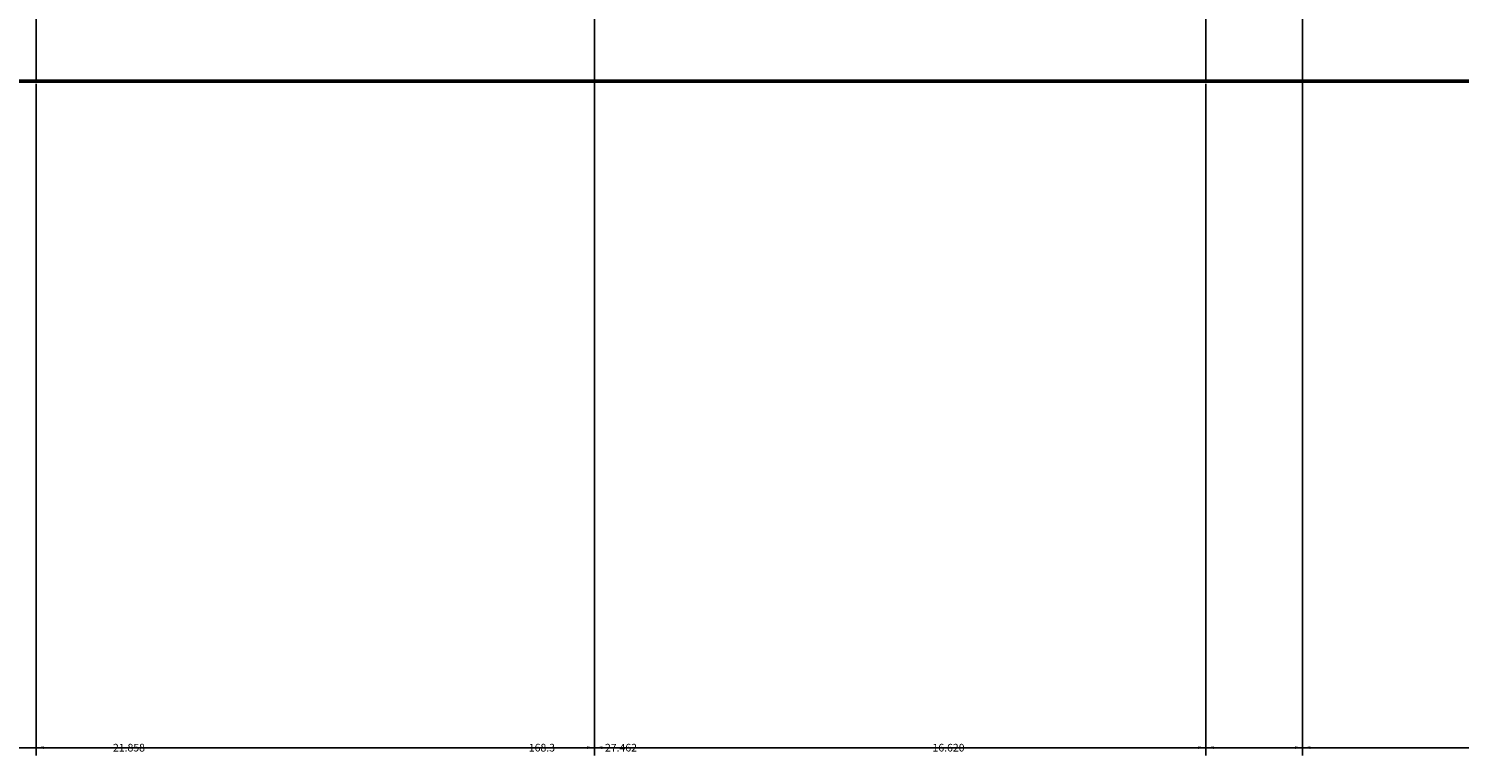
# Model space of a CAD drawing. Units: inches. Extents: x -117 to 121, y -77 to 40.
# Tile 19 of 45: x -6 to 28, y -77 to -60. Entities that reach past the tile are written whole.
import ezdxf

# ---------------------------------------------------------------- set-up
doc = ezdxf.new("R2010")
doc.units = ezdxf.units.IN
doc.header["$MEASUREMENT"] = 0
for name, color, linetype, lineweight in [('A-ANNO-DIMS', 2, 'Continuous', 18), ('A-ELEV', 7, 'Continuous', 25), ('A-ELEV-GRND', 7, 'Continuous', 50)]:
    doc.layers.add(name, color=color, linetype=linetype, lineweight=lineweight)
doc.styles.get("Standard").update_dxf_attribs({"font": 'arial.ttf'})
doc.dimstyles.get("Standard").update_dxf_attribs({"dimtxt": 0.18, "dimasz": 0.18, "dimexe": 0.18, "dimexo": 0.0625, "dimgap": 0.09, "dimtad": 0, "dimtih": 1, "dimtoh": 1, "dimdec": 4, "dimzin": 0, "dimdsep": 46, "dimtxsty": 'Standard', "dimcen": 0.09, "dimadec": 0, "dimazin": 0, "dimtfac": 1, "dimtdec": 4, "dimtofl": 0, "dimtmove": 0, "dimatfit": 3, "dimfxl": 1, "dimtolj": 1, "dimtzin": 0, "dimarcsym": 0})

# ---------------------------------------------------------------- blocks, each defined once
blk = doc.blocks.new('*D7')
at = {"layer": 'A-ANNO-DIMS', "color": 0, "lineweight": -2, "transparency": 16777216}
for p, q in [((-77.763, -61.431), (-77.763, -77.193)), ((90.549, -61.438), (90.549, -77.193)), ((-77.583, -77.013), (6.008, -77.013)), ((90.369, -77.013), (6.778, -77.013))]:
    blk.add_line(p, q, dxfattribs=at)
at = {"layer": 'A-ANNO-DIMS', "color": 0, "transparency": 16777216}
for points in [[(-77.583, -76.983), (-77.583, -77.043), (-77.763, -77.013)], [(90.369, -76.983), (90.369, -77.043), (90.549, -77.013)]]:
    blk.add_solid(points, dxfattribs=at)
at = {"layer": 'Defpoints', "color": 0, "transparency": 16777216}
for p in [(-77.763, -61.369), (90.549, -61.376), (90.549, -77.013)]:
    blk.add_point(p, dxfattribs=at)
at = {"layer": 'A-ANNO-DIMS', "color": 0, "transparency": 16777216, "insert": (6.393, -77.013), "char_height": 0.18, "attachment_point": 5}
blk.add_mtext('\\A1;168.3', dxfattribs=at)
blk = doc.blocks.new('*D13')
at = {"layer": 'A-ANNO-DIMS', "color": 0, "lineweight": -2, "transparency": 16777216}
for p, q in [((-2.663, 27.063), (-117.024, 27.063)), ((-116.844, 26.883), (-116.844, -16.974)), ((-116.844, -61.196), (-116.844, -17.338)), ((-106.096, -61.376), (-117.024, -61.376))]:
    blk.add_line(p, q, dxfattribs=at)
at = {"layer": 'A-ANNO-DIMS', "color": 0, "transparency": 16777216}
for points in [[(-116.874, 26.883), (-116.814, 26.883), (-116.844, 27.063)], [(-116.874, -61.196), (-116.814, -61.196), (-116.844, -61.376)]]:
    blk.add_solid(points, dxfattribs=at)
at = {"layer": 'Defpoints', "color": 0, "transparency": 16777216}
for p in [(-2.6, 27.063), (-116.844, -61.376), (-106.034, -61.376)]:
    blk.add_point(p, dxfattribs=at)
at = {"layer": 'A-ANNO-DIMS', "color": 0, "transparency": 16777216, "insert": (-116.844, -17.156), "char_height": 0.18, "attachment_point": 5}
blk.add_mtext('\\A1;88.44', dxfattribs=at)
blk = doc.blocks.new('*D25')
at = {"layer": 'A-ANNO-DIMS', "color": 0, "lineweight": -2, "transparency": 16777216}
for p, q in [((-5.482, -61.438), (-5.482, -77.193)), ((21.98, -61.438), (21.98, -77.193)), ((-5.302, -77.013), (7.784, -77.013)), ((21.8, -77.013), (8.713, -77.013))]:
    blk.add_line(p, q, dxfattribs=at)
at = {"layer": 'A-ANNO-DIMS', "color": 0, "transparency": 16777216}
for points in [[(-5.302, -76.983), (-5.302, -77.043), (-5.482, -77.013)], [(21.8, -76.983), (21.8, -77.043), (21.98, -77.013)]]:
    blk.add_solid(points, dxfattribs=at)
at = {"layer": 'Defpoints', "color": 0, "transparency": 16777216}
for p in [(-5.482, -61.376), (21.98, -61.376), (21.98, -77.013)]:
    blk.add_point(p, dxfattribs=at)
at = {"layer": 'A-ANNO-DIMS', "color": 0, "transparency": 16777216, "insert": (8.249, -77.013), "char_height": 0.18, "attachment_point": 5}
blk.add_mtext('\\A1;27.462', dxfattribs=at)
blk = doc.blocks.new('*D26')
at = {"layer": 'A-ANNO-DIMS', "color": 0, "lineweight": -2, "transparency": 16777216}
for p, q in [((21.98, -61.438), (21.98, -77.193)), ((40.68, -61.438), (40.68, -77.193)), ((22.16, -77.013), (30.892, -77.013)), ((40.5, -77.013), (31.768, -77.013))]:
    blk.add_line(p, q, dxfattribs=at)
at = {"layer": 'A-ANNO-DIMS', "color": 0, "transparency": 16777216}
for points in [[(22.16, -76.983), (22.16, -77.043), (21.98, -77.013)], [(40.5, -76.983), (40.5, -77.043), (40.68, -77.013)]]:
    blk.add_solid(points, dxfattribs=at)
at = {"layer": 'Defpoints', "color": 0, "transparency": 16777216}
for p in [(21.98, -61.376), (40.68, -61.376), (40.68, -77.013)]:
    blk.add_point(p, dxfattribs=at)
at = {"layer": 'A-ANNO-DIMS', "color": 0, "transparency": 16777216, "insert": (31.33, -77.013), "char_height": 0.18, "attachment_point": 5}
blk.add_mtext('\\A1;18.701', dxfattribs=at)
blk = doc.blocks.new('*D56')
at = {"layer": 'A-ANNO-DIMS', "color": 0, "lineweight": -2, "transparency": 16777216}
for p, q in [((-14.23, -7.853), (-14.23, -77.193)), ((7.628, -8.105), (7.628, -77.193)), ((-14.05, -77.013), (-3.766, -77.013)), ((7.448, -77.013), (-2.835, -77.013))]:
    blk.add_line(p, q, dxfattribs=at)
at = {"layer": 'A-ANNO-DIMS', "color": 0, "transparency": 16777216}
for points in [[(-14.05, -76.983), (-14.05, -77.043), (-14.23, -77.013)], [(7.448, -76.983), (7.448, -77.043), (7.628, -77.013)]]:
    blk.add_solid(points, dxfattribs=at)
at = {"layer": 'Defpoints', "color": 0, "transparency": 16777216}
for p in [(-14.23, -7.791), (7.628, -8.042), (7.628, -77.013)]:
    blk.add_point(p, dxfattribs=at)
at = {"layer": 'A-ANNO-DIMS', "color": 0, "transparency": 16777216, "insert": (-3.301, -77.013), "char_height": 0.18, "attachment_point": 5}
blk.add_mtext('\\A1;21.858', dxfattribs=at)
blk = doc.blocks.new('*D57')
at = {"layer": 'A-ANNO-DIMS', "color": 0, "lineweight": -2, "transparency": 16777216}
for p, q in [((7.628, -8.105), (7.628, -77.193)), ((24.248, -8.105), (24.248, -77.193)), ((7.808, -77.013), (15.483, -77.013)), ((24.068, -77.013), (16.393, -77.013))]:
    blk.add_line(p, q, dxfattribs=at)
at = {"layer": 'A-ANNO-DIMS', "color": 0, "transparency": 16777216}
for points in [[(7.808, -76.983), (7.808, -77.043), (7.628, -77.013)], [(24.068, -76.983), (24.068, -77.043), (24.248, -77.013)]]:
    blk.add_solid(points, dxfattribs=at)
at = {"layer": 'Defpoints', "color": 0, "transparency": 16777216}
for p in [(7.628, -8.042), (24.248, -8.042), (24.248, -77.013)]:
    blk.add_point(p, dxfattribs=at)
at = {"layer": 'A-ANNO-DIMS', "color": 0, "transparency": 16777216, "insert": (15.938, -77.013), "char_height": 0.18, "attachment_point": 5}
blk.add_mtext('\\A1;16.620', dxfattribs=at)
blk = doc.blocks.new('*D58')
at = {"layer": 'A-ANNO-DIMS', "color": 0, "lineweight": -2, "transparency": 16777216}
for p, q in [((57.61, -7.947), (57.61, -77.193)), ((24.248, -8.105), (24.248, -77.193)), ((24.428, -77.013), (40.467, -77.013)), ((57.43, -77.013), (41.392, -77.013))]:
    blk.add_line(p, q, dxfattribs=at)
at = {"layer": 'A-ANNO-DIMS', "color": 0, "transparency": 16777216}
for points in [[(24.428, -76.983), (24.428, -77.043), (24.248, -77.013)], [(57.43, -76.983), (57.43, -77.043), (57.61, -77.013)]]:
    blk.add_solid(points, dxfattribs=at)
at = {"layer": 'Defpoints', "color": 0, "transparency": 16777216}
for p in [(24.248, -8.042), (57.61, -7.885), (57.61, -77.013)]:
    blk.add_point(p, dxfattribs=at)
at = {"layer": 'A-ANNO-DIMS', "color": 0, "transparency": 16777216, "insert": (40.929, -77.013), "char_height": 0.18, "attachment_point": 5}
blk.add_mtext('\\A1;33.362', dxfattribs=at)

msp = doc.modelspace()

# ---------------------------------------------------------------- linework, layer by layer
at = {"layer": 'A-ELEV'}
for p, q in [((-5.4823, -31.9617), (-5.4823, -61.3756)), ((21.9795, -43.6334), (21.9795, -61.3756))]:
    msp.add_line(p, q, dxfattribs=at)
at = {"layer": 'A-ELEV-GRND'}
msp.add_line((90.5486, -61.3756), (-87.9273, -61.3756), dxfattribs=at)

# ---------------------------------------------------------------- dimensions: what is measured, and where the dimension line sits
at = {"layer": 'A-ANNO-DIMS'}
dim = msp.add_linear_dim(base=(-116.8438, -61.3756), p1=(-2.6001, 27.0634), p2=(-106.0338, -61.3756), angle=90, dimstyle='Standard', override={"dimdec": 2, "dimlfac": 1, "dimrnd": 0, "dimzin": 0, "dimdsep": 46, "dimlunit": 2}, dxfattribs=at)
dim.commit()
dim.dimension.update_dxf_attribs({"geometry": '*D13', "text_midpoint": (-116.8438, -17.1561)})
for base, p1, p2, override, picture, middle in [((7.6284, -77.0135), (-14.2298, -7.7907), (7.6284, -8.0421), {"dimdec": 3, "dimlfac": 1, "dimrnd": 0, "dimzin": 0, "dimdsep": 46, "dimlunit": 2}, '*D56', (-3.3007, -77.0135)), ((24.2481, -77.0135), (7.6284, -8.0421), (24.2481, -8.0421), {"dimdec": 3, "dimlfac": 1, "dimrnd": 0, "dimzin": 0, "dimdsep": 46, "dimlunit": 2}, '*D57', (15.9383, -77.0135)), ((57.6104, -77.0135), (24.2481, -8.0421), (57.6104, -7.8846), {"dimdec": 3, "dimlfac": 1, "dimrnd": 0, "dimzin": 0, "dimdsep": 46, "dimlunit": 2}, '*D58', (40.9293, -77.0135)), ((90.5486, -77.0135), (-77.7631, -61.3689), (90.5486, -61.3756), {"dimdec": 1, "dimlfac": 1, "dimrnd": 0, "dimzin": 0, "dimdsep": 46, "dimlunit": 2}, '*D7', (6.3928, -77.0135)), ((21.9795, -77.0135), (-5.4823, -61.3756), (21.9795, -61.3756), {"dimdec": 3, "dimlfac": 1, "dimrnd": 0, "dimzin": 0, "dimdsep": 46, "dimlunit": 2}, '*D25', (8.2486, -77.0135)), ((40.6802, -77.0135), (21.9795, -61.3756), (40.6802, -61.3756), {"dimdec": 3, "dimlfac": 1, "dimrnd": 0, "dimzin": 0, "dimdsep": 46, "dimlunit": 2}, '*D26', (31.3299, -77.0135))]:
    dim = msp.add_linear_dim(base=base, p1=p1, p2=p2, dimstyle='Standard', override=override, dxfattribs=at)
    dim.commit()
    dim.dimension.update_dxf_attribs({"geometry": picture, "text_midpoint": middle})

doc.saveas('drawing.dxf')
